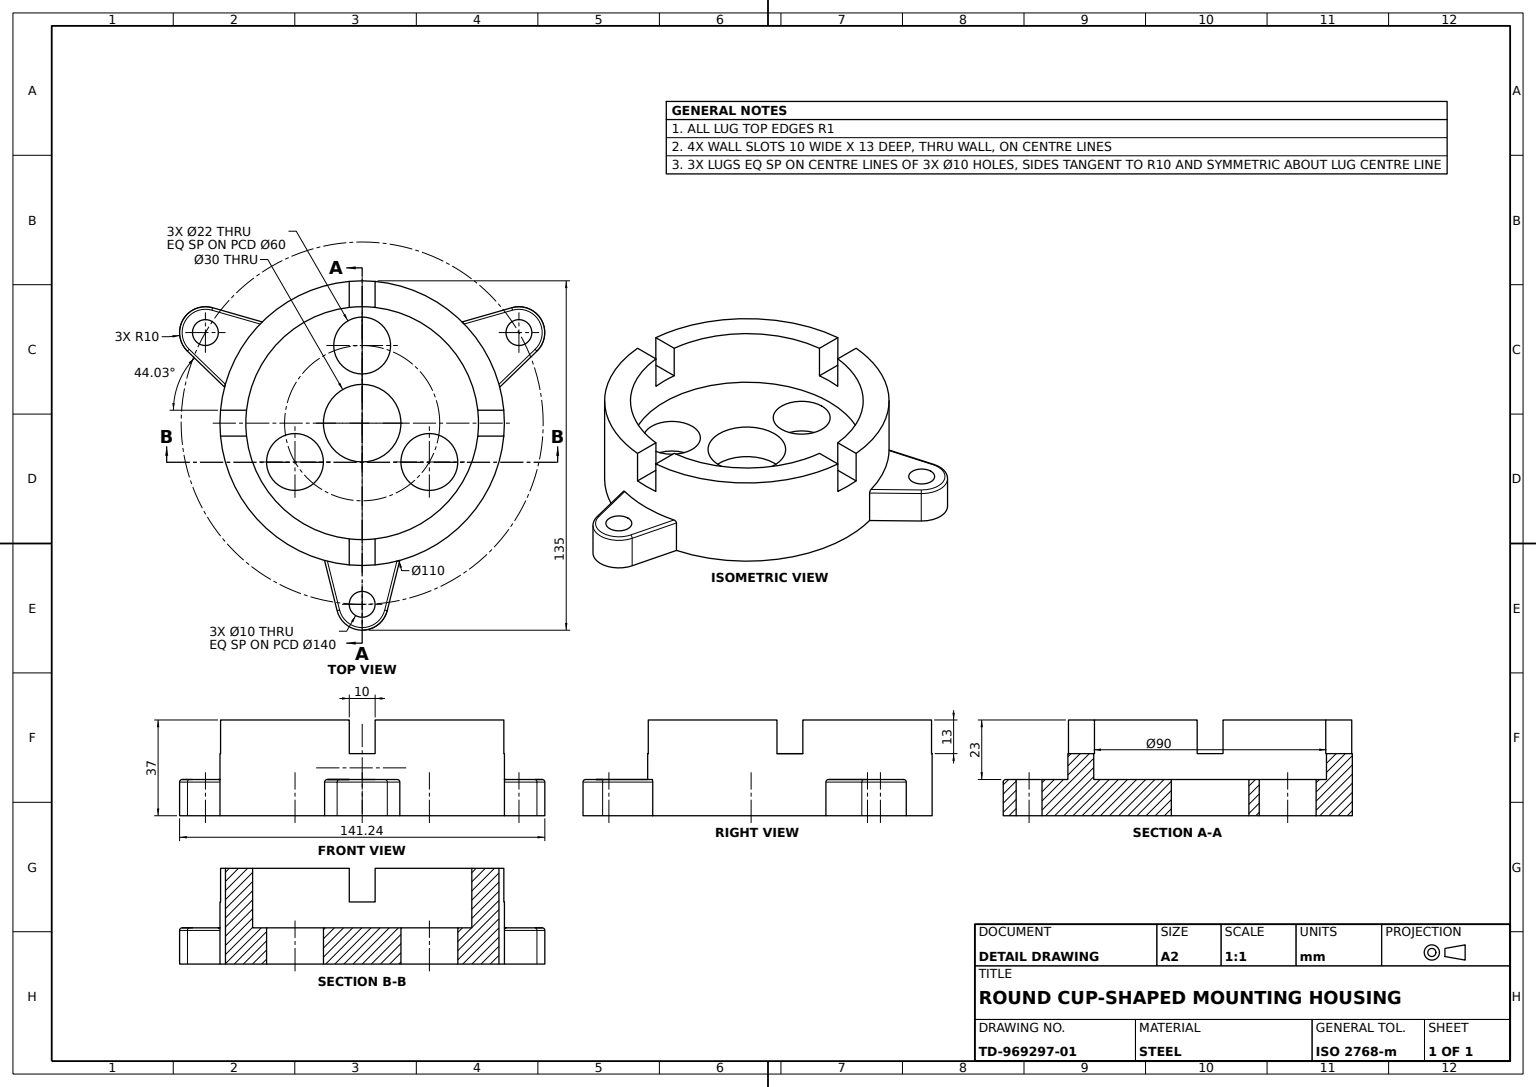
SolidWorks part; units mm, degrees
material "Plain Carbon Steel"
ref_plane "Front Plane" through (0, 0, 0) normal (0, 0, 1) x (1, 0, 0)
ref_plane "Top Plane" through (0, 0, 0) normal (0, 1, 0) x (1, 0, 0)
ref_plane "Right Plane" through (0, 0, 0) normal (1, 0, 0) x (0, 0, -1)
sketch "Flange Profile Sketch" plane through (0, 0, 0) normal (0, 1, 0) x (1, 0, 0)
  line L1 (9.7018, -72.4238) -> (14.5438, -53.0422)
  line L2 (-9.7018, -72.4238) -> (-14.5438, -53.0422)
  line L4 (-57.8699, 44.6139) -> (-38.664, 39.1164)
  line L5 (-67.5717, 27.8099) -> (-53.2078, 13.9258)
  line L6 (67.5717, 27.8099) -> (53.2078, 13.9258)
  line L7 (57.8699, 44.6139) -> (38.664, 39.1164)
  arc A0 (-53.2078, 13.9258) -> (-14.5438, -53.0422) centre (0, 0) ccw
  circle A1 centre (0, 0) radius 45
  arc A5 (-9.7018, -72.4238) -> (9.7018, -72.4238) centre (0, -70) ccw
  circle A6 centre (0, -70) radius 5
  arc A7 (-57.8699, 44.6139) -> (-67.5717, 27.8099) centre (-60.6218, 35) ccw
  circle A8 centre (-60.6218, 35) radius 5
  arc A9 (67.5717, 27.8099) -> (57.8699, 44.6139) centre (60.6218, 35) ccw
  circle A10 centre (60.6218, 35) radius 5
  arc A11 (38.664, 39.1164) -> (-38.664, 39.1164) centre (0, 0) ccw
  arc A12 (14.5438, -53.0422) -> (53.2078, 13.9258) centre (0, 0) ccw
  circle A14 centre (0, 30) radius 11
  circle A15 centre (25.9808, -15) radius 11
  circle A16 centre (-25.9808, -15) radius 11
  circle A17 centre (0, 0) radius 15
  dimension "D1" = 110
  dimension "D2" = 90
  dimension "D3" = 10
  dimension "D5" = 3
  dimension "D4" = 10
  dimension "D6" = 30
  dimension "D7" = 22
  dimension "D9" = 6.95
  dimension "D10" = 14.3639
  dimension "D11" = 41.591
  dimension "D12" = 14.6139
  dimension "D8" = 3
extrude "Mounting Flange 3 Lugs" add sketch "Flange Profile Sketch" along normal blind 14 contours L1 A12 L6 A9 L7 A11 L4 A7 L5 A0 L2 A5 A1 A6 A8 A10 | A1 A17 A16 A15 A14
fillet "Flange Edge Fillet R1" radius 1 9 edges at (60.3898, 14, -20.8678) (69.282, 14, -40) (12.1228, 14, 62.733) (0, 14, 80) (-60.3898, 14, -20.8678) (-69.282, 14, -40) (48.267, 14, -41.8652) (-12.1228, 14, 62.733) (-48.267, 14, -41.8652)
sketch "Bearing Wall Sketch" plane through (0, 14, 0) normal (0, 1, 0) x (1, 0, 0)
  circle A0 centre (0, 0) radius 55
  circle A1 centre (0, 0) radius 45
  dimension "D1" = 110
  dimension "D2" = 90
extrude "Bearing Wall Ø110" add sketch "Bearing Wall Sketch" along normal blind 23
sketch "Wall Slots Sketch" plane through (0, 37, 0) normal (0, 1, 0) x (1, 0, 0)
  line L0 (-44.7214, 5) -> (-54.7723, 5)
  line L1 (-5, -44.7214) -> (-5, -54.7723)
  line L2 (5, -44.7214) -> (5, -54.7723)
  line L3 (-44.7214, -5) -> (-54.7723, -5)
  line L4 (5, 44.7214) -> (5, 54.7723)
  line L5 (-5, 44.7214) -> (-5, 54.7723)
  line L6 (44.7214, -5) -> (54.7723, -5)
  line L7 (44.7214, 5) -> (54.7723, 5)
  circle A0 centre (0, 0) radius 45
  circle A1 centre (0, 0) radius 55
  circle A2 centre (0, 0) radius 55 construction
  point P4 (0, -55)
  point P5 (-5, 0)
  point P6 (-5, -55)
  point P7 (5, 0)
  point P8 (5, -55)
  circle M2 centre (0, 0) radius 55
  circle M3 centre (0, 0) radius 45
  dimension "D1" = 110
  dimension "D2" = 90
  dimension "D3" = 4
  dimension "D4" = 5
extrude "Wall Slots 4x" cut sketch "Wall Slots Sketch" against normal blind 13 contours L3 L0 M3 M2 | L5 L4 M3 M2 | L7 L6 M3 M2 | L2 L1 M3 M2
